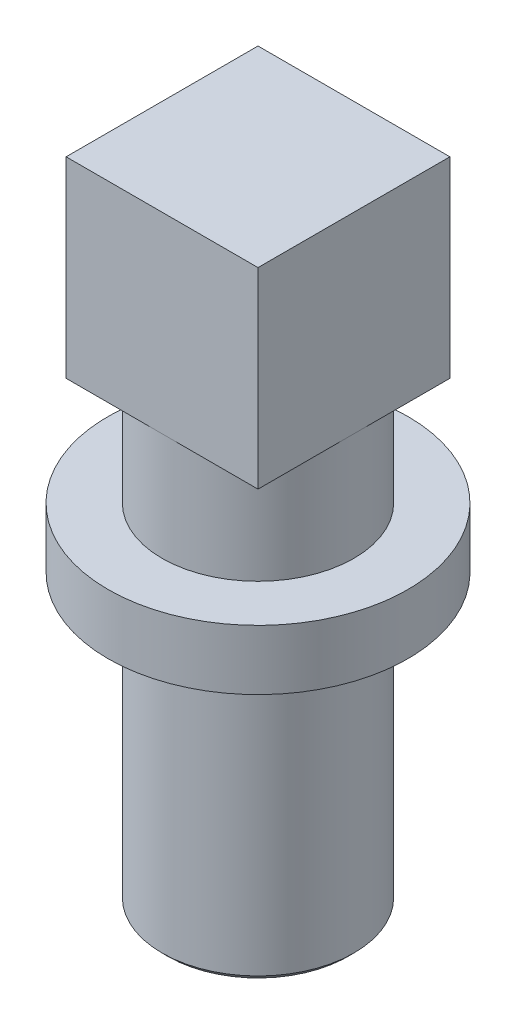
ISO-10303-21;
HEADER;
FILE_DESCRIPTION(('STEP AP214'),'2;1');
FILE_NAME('part.step','',(''),(''),'','','');
FILE_SCHEMA(('AUTOMOTIVE_DESIGN { 1 0 10303 214 1 1 1 1 }'));
ENDSEC;
DATA;
#1=APPLICATION_CONTEXT('core data for automotive mechanical design processes');
#2=APPLICATION_PROTOCOL_DEFINITION('international standard','automotive_design',2000,#1);
#3=PRODUCT_CONTEXT('',#1,'mechanical');
#4=PRODUCT('Part','Part','',(#3));
#5=PRODUCT_RELATED_PRODUCT_CATEGORY('part','',(#4));
#6=PRODUCT_DEFINITION_FORMATION('','',#4);
#7=PRODUCT_DEFINITION_CONTEXT('part definition',#1,'design');
#8=PRODUCT_DEFINITION('design','',#6,#7);
#9=PRODUCT_DEFINITION_SHAPE('','',#8);
#10=(LENGTH_UNIT() NAMED_UNIT(*) SI_UNIT(.MILLI.,.METRE.));
#11=(NAMED_UNIT(*) PLANE_ANGLE_UNIT() SI_UNIT($,.RADIAN.));
#12=(NAMED_UNIT(*) SI_UNIT($,.STERADIAN.) SOLID_ANGLE_UNIT());
#13=UNCERTAINTY_MEASURE_WITH_UNIT(LENGTH_MEASURE(1.E-05),#10,'distance_accuracy_value','');
#14=(GEOMETRIC_REPRESENTATION_CONTEXT(3) GLOBAL_UNCERTAINTY_ASSIGNED_CONTEXT((#13)) GLOBAL_UNIT_ASSIGNED_CONTEXT((#10,
#11,#12)) REPRESENTATION_CONTEXT('',''));
#15=CARTESIAN_POINT('',(0.,0.,0.));
#16=DIRECTION('',(0.,0.,1.));
#17=DIRECTION('',(1.,0.,0.));
#18=AXIS2_PLACEMENT_3D('',#15,#16,#17);
#19=CARTESIAN_POINT('',(0.,24.,0.));
#20=DIRECTION('',(0.,-1.,0.));
#21=DIRECTION('',(0.,0.,-1.));
#22=AXIS2_PLACEMENT_3D('',#19,#20,#21);
#23=CYLINDRICAL_SURFACE('',#22,8.);
#24=CARTESIAN_POINT('',(0.,0.500000000000004,0.));
#25=DIRECTION('',(0.,1.,0.));
#26=DIRECTION('',(0.,0.,1.));
#27=AXIS2_PLACEMENT_3D('',#24,#25,#26);
#28=CIRCLE('',#27,8.);
#29=CARTESIAN_POINT('',(0.,0.500000000000004,8.));
#30=VERTEX_POINT('',#29);
#31=EDGE_CURVE('E138',#30,#30,#28,.T.);
#32=ORIENTED_EDGE('',*,*,#31,.T.);
#33=EDGE_LOOP('',(#32));
#34=FACE_BOUND('',#33,.T.);
#35=CARTESIAN_POINT('',(0.,24.,0.));
#36=DIRECTION('',(0.,1.,0.));
#37=DIRECTION('',(0.,0.,1.));
#38=AXIS2_PLACEMENT_3D('',#35,#36,#37);
#39=CIRCLE('',#38,8.);
#40=CARTESIAN_POINT('',(0.,24.,8.));
#41=VERTEX_POINT('',#40);
#42=EDGE_CURVE('E134',#41,#41,#39,.T.);
#43=ORIENTED_EDGE('',*,*,#42,.F.);
#44=EDGE_LOOP('',(#43));
#45=FACE_BOUND('',#44,.T.);
#46=ADVANCED_FACE('F41',(#34,#45),#23,.T.);
#47=CARTESIAN_POINT('',(0.,0.,0.));
#48=DIRECTION('',(0.,1.,0.));
#49=DIRECTION('',(0.,0.,1.));
#50=AXIS2_PLACEMENT_3D('',#47,#48,#49);
#51=PLANE('',#50);
#52=CARTESIAN_POINT('',(0.,0.,0.));
#53=DIRECTION('',(0.,1.,0.));
#54=DIRECTION('',(0.,0.,1.));
#55=AXIS2_PLACEMENT_3D('',#52,#53,#54);
#56=CIRCLE('',#55,7.5);
#57=CARTESIAN_POINT('',(0.,0.,7.5));
#58=VERTEX_POINT('',#57);
#59=EDGE_CURVE('E46',#58,#58,#56,.F.);
#60=ORIENTED_EDGE('',*,*,#59,.T.);
#61=EDGE_LOOP('',(#60));
#62=FACE_BOUND('',#61,.T.);
#63=ADVANCED_FACE('F144',(#62),#51,.F.);
#64=CARTESIAN_POINT('',(0.,0.500000000000004,0.));
#65=DIRECTION('',(0.,1.,0.));
#66=DIRECTION('',(0.,0.,1.));
#67=AXIS2_PLACEMENT_3D('',#64,#65,#66);
#68=CONICAL_SURFACE('',#67,8.,0.785398163397448);
#69=ORIENTED_EDGE('',*,*,#59,.F.);
#70=EDGE_LOOP('',(#69));
#71=FACE_BOUND('',#70,.T.);
#72=ORIENTED_EDGE('',*,*,#31,.F.);
#73=EDGE_LOOP('',(#72));
#74=FACE_BOUND('',#73,.T.);
#75=ADVANCED_FACE('F42',(#71,#74),#68,.T.);
#76=CARTESIAN_POINT('',(0.,29.,0.));
#77=DIRECTION('',(0.,-1.,0.));
#78=DIRECTION('',(0.,0.,-1.));
#79=AXIS2_PLACEMENT_3D('',#76,#77,#78);
#80=CYLINDRICAL_SURFACE('',#79,12.5);
#81=CARTESIAN_POINT('',(0.,29.,0.));
#82=DIRECTION('',(0.,1.,0.));
#83=DIRECTION('',(0.,0.,1.));
#84=AXIS2_PLACEMENT_3D('',#81,#82,#83);
#85=CIRCLE('',#84,12.5);
#86=CARTESIAN_POINT('',(0.,29.,12.5));
#87=VERTEX_POINT('',#86);
#88=EDGE_CURVE('E132',#87,#87,#85,.T.);
#89=ORIENTED_EDGE('',*,*,#88,.F.);
#90=EDGE_LOOP('',(#89));
#91=FACE_BOUND('',#90,.T.);
#92=CARTESIAN_POINT('',(0.,24.,0.));
#93=DIRECTION('',(0.,1.,0.));
#94=DIRECTION('',(0.,0.,1.));
#95=AXIS2_PLACEMENT_3D('',#92,#93,#94);
#96=CIRCLE('',#95,12.5);
#97=CARTESIAN_POINT('',(0.,24.,12.5));
#98=VERTEX_POINT('',#97);
#99=EDGE_CURVE('E126',#98,#98,#96,.T.);
#100=ORIENTED_EDGE('',*,*,#99,.T.);
#101=EDGE_LOOP('',(#100));
#102=FACE_BOUND('',#101,.T.);
#103=ADVANCED_FACE('F149',(#91,#102),#80,.T.);
#104=CARTESIAN_POINT('',(0.,29.,0.));
#105=DIRECTION('',(0.,1.,0.));
#106=DIRECTION('',(0.,0.,1.));
#107=AXIS2_PLACEMENT_3D('',#104,#105,#106);
#108=PLANE('',#107);
#109=CARTESIAN_POINT('',(0.,29.,0.));
#110=DIRECTION('',(0.,1.,0.));
#111=DIRECTION('',(0.,0.,1.));
#112=AXIS2_PLACEMENT_3D('',#109,#110,#111);
#113=CIRCLE('',#112,8.);
#114=CARTESIAN_POINT('',(0.,29.,8.));
#115=VERTEX_POINT('',#114);
#116=EDGE_CURVE('E11',#115,#115,#113,.T.);
#117=ORIENTED_EDGE('',*,*,#116,.F.);
#118=EDGE_LOOP('',(#117));
#119=FACE_BOUND('',#118,.T.);
#120=ORIENTED_EDGE('',*,*,#88,.T.);
#121=EDGE_LOOP('',(#120));
#122=FACE_BOUND('',#121,.T.);
#123=ADVANCED_FACE('F152',(#119,#122),#108,.T.);
#124=CARTESIAN_POINT('',(0.,24.,0.));
#125=DIRECTION('',(0.,1.,0.));
#126=DIRECTION('',(0.,0.,1.));
#127=AXIS2_PLACEMENT_3D('',#124,#125,#126);
#128=PLANE('',#127);
#129=ORIENTED_EDGE('',*,*,#42,.T.);
#130=EDGE_LOOP('',(#129));
#131=FACE_BOUND('',#130,.T.);
#132=ORIENTED_EDGE('',*,*,#99,.F.);
#133=EDGE_LOOP('',(#132));
#134=FACE_BOUND('',#133,.T.);
#135=ADVANCED_FACE('F162',(#131,#134),#128,.F.);
#136=CARTESIAN_POINT('',(0.,38.,0.));
#137=DIRECTION('',(0.,-1.,0.));
#138=DIRECTION('',(0.,0.,-1.));
#139=AXIS2_PLACEMENT_3D('',#136,#137,#138);
#140=CYLINDRICAL_SURFACE('',#139,8.);
#141=CARTESIAN_POINT('',(0.,38.,0.));
#142=DIRECTION('',(0.,1.,0.));
#143=DIRECTION('',(0.,0.,1.));
#144=AXIS2_PLACEMENT_3D('',#141,#142,#143);
#145=CIRCLE('',#144,8.);
#146=CARTESIAN_POINT('',(0.,38.,8.));
#147=VERTEX_POINT('',#146);
#148=CARTESIAN_POINT('',(8.,38.,0.));
#149=VERTEX_POINT('',#148);
#150=EDGE_CURVE('E123',#147,#149,#145,.T.);
#151=ORIENTED_EDGE('',*,*,#150,.F.);
#152=CARTESIAN_POINT('',(-8.,38.,0.));
#153=VERTEX_POINT('',#152);
#154=EDGE_CURVE('E59',#153,#147,#145,.T.);
#155=ORIENTED_EDGE('',*,*,#154,.F.);
#156=CARTESIAN_POINT('',(0.,38.,-8.));
#157=VERTEX_POINT('',#156);
#158=EDGE_CURVE('E65',#157,#153,#145,.T.);
#159=ORIENTED_EDGE('',*,*,#158,.F.);
#160=EDGE_CURVE('E129',#149,#157,#145,.T.);
#161=ORIENTED_EDGE('',*,*,#160,.F.);
#162=EDGE_LOOP('',(#151,#155,#159,#161));
#163=FACE_BOUND('',#162,.T.);
#164=ORIENTED_EDGE('',*,*,#116,.T.);
#165=EDGE_LOOP('',(#164));
#166=FACE_BOUND('',#165,.T.);
#167=ADVANCED_FACE('F167',(#163,#166),#140,.T.);
#168=CARTESIAN_POINT('',(0.,38.,0.));
#169=DIRECTION('',(0.,-1.,0.));
#170=DIRECTION('',(0.,0.,-1.));
#171=AXIS2_PLACEMENT_3D('',#168,#169,#170);
#172=PLANE('',#171);
#173=DIRECTION('',(1.,0.,0.));
#174=VECTOR('',#173,1.);
#175=CARTESIAN_POINT('',(-8.,38.,8.));
#176=LINE('',#175,#174);
#177=CARTESIAN_POINT('',(8.,38.,8.));
#178=VERTEX_POINT('',#177);
#179=EDGE_CURVE('E291',#147,#178,#176,.T.);
#180=ORIENTED_EDGE('',*,*,#179,.F.);
#181=ORIENTED_EDGE('',*,*,#150,.T.);
#182=DIRECTION('',(0.,0.,-1.));
#183=VECTOR('',#182,1.);
#184=CARTESIAN_POINT('',(8.,38.,8.));
#185=LINE('',#184,#183);
#186=EDGE_CURVE('E293',#178,#149,#185,.T.);
#187=ORIENTED_EDGE('',*,*,#186,.F.);
#188=EDGE_LOOP('',(#180,#181,#187));
#189=FACE_BOUND('',#188,.T.);
#190=ADVANCED_FACE('F173',(#189),#172,.T.);
#191=CARTESIAN_POINT('',(8.,38.,-8.));
#192=VERTEX_POINT('',#191);
#193=EDGE_CURVE('E119',#149,#192,#185,.T.);
#194=ORIENTED_EDGE('',*,*,#193,.F.);
#195=ORIENTED_EDGE('',*,*,#160,.T.);
#196=DIRECTION('',(-1.,0.,0.));
#197=VECTOR('',#196,1.);
#198=CARTESIAN_POINT('',(-8.,38.,-8.));
#199=LINE('',#198,#197);
#200=EDGE_CURVE('E309',#192,#157,#199,.T.);
#201=ORIENTED_EDGE('',*,*,#200,.F.);
#202=EDGE_LOOP('',(#194,#195,#201));
#203=FACE_BOUND('',#202,.T.);
#204=ADVANCED_FACE('F226',(#203),#172,.T.);
#205=CARTESIAN_POINT('',(-8.,38.,-8.));
#206=VERTEX_POINT('',#205);
#207=EDGE_CURVE('E310',#157,#206,#199,.T.);
#208=ORIENTED_EDGE('',*,*,#207,.F.);
#209=ORIENTED_EDGE('',*,*,#158,.T.);
#210=DIRECTION('',(0.,0.,1.));
#211=VECTOR('',#210,1.);
#212=CARTESIAN_POINT('',(-8.,38.,8.));
#213=LINE('',#212,#211);
#214=EDGE_CURVE('E297',#206,#153,#213,.T.);
#215=ORIENTED_EDGE('',*,*,#214,.F.);
#216=EDGE_LOOP('',(#208,#209,#215));
#217=FACE_BOUND('',#216,.T.);
#218=ADVANCED_FACE('F177',(#217),#172,.T.);
#219=CARTESIAN_POINT('',(8.,54.,8.));
#220=DIRECTION('',(-1.,0.,0.));
#221=DIRECTION('',(0.,0.,1.));
#222=AXIS2_PLACEMENT_3D('',#219,#220,#221);
#223=PLANE('',#222);
#224=ORIENTED_EDGE('',*,*,#186,.T.);
#225=ORIENTED_EDGE('',*,*,#193,.T.);
#226=DIRECTION('',(0.,-1.,0.));
#227=VECTOR('',#226,1.);
#228=CARTESIAN_POINT('',(8.,54.,-8.));
#229=LINE('',#228,#227);
#230=CARTESIAN_POINT('',(8.,54.,-8.));
#231=VERTEX_POINT('',#230);
#232=EDGE_CURVE('E97',#231,#192,#229,.T.);
#233=ORIENTED_EDGE('',*,*,#232,.F.);
#234=DIRECTION('',(0.,0.,-1.));
#235=VECTOR('',#234,1.);
#236=CARTESIAN_POINT('',(8.,54.,8.));
#237=LINE('',#236,#235);
#238=CARTESIAN_POINT('',(8.,54.,8.));
#239=VERTEX_POINT('',#238);
#240=EDGE_CURVE('E104',#239,#231,#237,.T.);
#241=ORIENTED_EDGE('',*,*,#240,.F.);
#242=DIRECTION('',(0.,-1.,0.));
#243=VECTOR('',#242,1.);
#244=CARTESIAN_POINT('',(8.,54.,8.));
#245=LINE('',#244,#243);
#246=EDGE_CURVE('E301',#239,#178,#245,.T.);
#247=ORIENTED_EDGE('',*,*,#246,.T.);
#248=EDGE_LOOP('',(#224,#225,#233,#241,#247));
#249=FACE_BOUND('',#248,.T.);
#250=ADVANCED_FACE('F120',(#249),#223,.F.);
#251=CARTESIAN_POINT('',(-8.,54.,-8.));
#252=DIRECTION('',(0.,0.,1.));
#253=DIRECTION('',(1.,0.,0.));
#254=AXIS2_PLACEMENT_3D('',#251,#252,#253);
#255=PLANE('',#254);
#256=ORIENTED_EDGE('',*,*,#200,.T.);
#257=ORIENTED_EDGE('',*,*,#207,.T.);
#258=DIRECTION('',(0.,-1.,0.));
#259=VECTOR('',#258,1.);
#260=CARTESIAN_POINT('',(-8.,54.,-8.));
#261=LINE('',#260,#259);
#262=CARTESIAN_POINT('',(-8.,54.,-8.));
#263=VERTEX_POINT('',#262);
#264=EDGE_CURVE('E101',#263,#206,#261,.T.);
#265=ORIENTED_EDGE('',*,*,#264,.F.);
#266=DIRECTION('',(-1.,0.,0.));
#267=VECTOR('',#266,1.);
#268=CARTESIAN_POINT('',(-8.,54.,-8.));
#269=LINE('',#268,#267);
#270=EDGE_CURVE('E94',#231,#263,#269,.T.);
#271=ORIENTED_EDGE('',*,*,#270,.F.);
#272=ORIENTED_EDGE('',*,*,#232,.T.);
#273=EDGE_LOOP('',(#256,#257,#265,#271,#272));
#274=FACE_BOUND('',#273,.T.);
#275=ADVANCED_FACE('F100',(#274),#255,.F.);
#276=CARTESIAN_POINT('',(-8.,54.,8.));
#277=DIRECTION('',(1.,0.,0.));
#278=DIRECTION('',(0.,0.,-1.));
#279=AXIS2_PLACEMENT_3D('',#276,#277,#278);
#280=PLANE('',#279);
#281=ORIENTED_EDGE('',*,*,#214,.T.);
#282=CARTESIAN_POINT('',(-8.,38.,8.));
#283=VERTEX_POINT('',#282);
#284=EDGE_CURVE('E313',#153,#283,#213,.T.);
#285=ORIENTED_EDGE('',*,*,#284,.T.);
#286=DIRECTION('',(0.,-1.,0.));
#287=VECTOR('',#286,1.);
#288=CARTESIAN_POINT('',(-8.,54.,8.));
#289=LINE('',#288,#287);
#290=CARTESIAN_POINT('',(-8.,54.,8.));
#291=VERTEX_POINT('',#290);
#292=EDGE_CURVE('E124',#291,#283,#289,.T.);
#293=ORIENTED_EDGE('',*,*,#292,.F.);
#294=DIRECTION('',(0.,0.,1.));
#295=VECTOR('',#294,1.);
#296=CARTESIAN_POINT('',(-8.,54.,8.));
#297=LINE('',#296,#295);
#298=EDGE_CURVE('E102',#263,#291,#297,.T.);
#299=ORIENTED_EDGE('',*,*,#298,.F.);
#300=ORIENTED_EDGE('',*,*,#264,.T.);
#301=EDGE_LOOP('',(#281,#285,#293,#299,#300));
#302=FACE_BOUND('',#301,.T.);
#303=ADVANCED_FACE('F179',(#302),#280,.F.);
#304=CARTESIAN_POINT('',(-8.,54.,8.));
#305=DIRECTION('',(0.,0.,-1.));
#306=DIRECTION('',(-1.,0.,0.));
#307=AXIS2_PLACEMENT_3D('',#304,#305,#306);
#308=PLANE('',#307);
#309=EDGE_CURVE('E111',#283,#147,#176,.T.);
#310=ORIENTED_EDGE('',*,*,#309,.T.);
#311=ORIENTED_EDGE('',*,*,#179,.T.);
#312=ORIENTED_EDGE('',*,*,#246,.F.);
#313=DIRECTION('',(1.,0.,0.));
#314=VECTOR('',#313,1.);
#315=CARTESIAN_POINT('',(-8.,54.,8.));
#316=LINE('',#315,#314);
#317=EDGE_CURVE('E109',#291,#239,#316,.T.);
#318=ORIENTED_EDGE('',*,*,#317,.F.);
#319=ORIENTED_EDGE('',*,*,#292,.T.);
#320=EDGE_LOOP('',(#310,#311,#312,#318,#319));
#321=FACE_BOUND('',#320,.T.);
#322=ADVANCED_FACE('F185',(#321),#308,.F.);
#323=CARTESIAN_POINT('',(0.,54.,0.));
#324=DIRECTION('',(0.,-1.,0.));
#325=DIRECTION('',(0.,0.,-1.));
#326=AXIS2_PLACEMENT_3D('',#323,#324,#325);
#327=PLANE('',#326);
#328=ORIENTED_EDGE('',*,*,#240,.T.);
#329=ORIENTED_EDGE('',*,*,#270,.T.);
#330=ORIENTED_EDGE('',*,*,#298,.T.);
#331=ORIENTED_EDGE('',*,*,#317,.T.);
#332=EDGE_LOOP('',(#328,#329,#330,#331));
#333=FACE_BOUND('',#332,.T.);
#334=ADVANCED_FACE('F107',(#333),#327,.F.);
#335=ORIENTED_EDGE('',*,*,#284,.F.);
#336=ORIENTED_EDGE('',*,*,#154,.T.);
#337=ORIENTED_EDGE('',*,*,#309,.F.);
#338=EDGE_LOOP('',(#335,#336,#337));
#339=FACE_BOUND('',#338,.T.);
#340=ADVANCED_FACE('F190',(#339),#172,.T.);
#341=CLOSED_SHELL('',(#46,#63,#75,#103,#123,#135,#167,#190,#204,#218,#250,#275,#303,#322,#334,#340));
#342=MANIFOLD_SOLID_BREP('B2',#341);
#343=ADVANCED_BREP_SHAPE_REPRESENTATION('',(#18,#342),#14);
#344=SHAPE_DEFINITION_REPRESENTATION(#9,#343);
ENDSEC;
END-ISO-10303-21;
